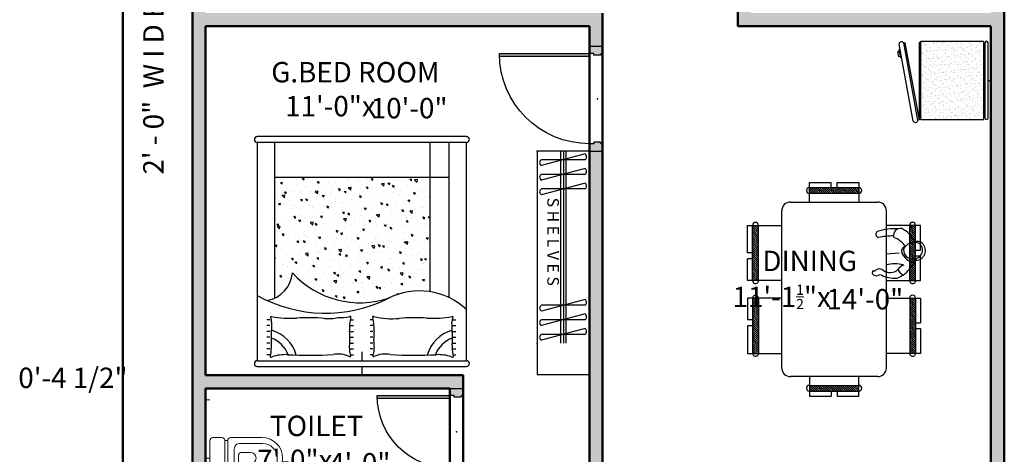
# Model space of a CAD drawing. Units: inches. Extents: x 4508 to 5907, y 877 to 1592.
# Tile 3 of 20: x 4536 to 4874, y 1182 to 1331. Entities that reach past the tile are written whole.
import ezdxf

# ---------------------------------------------------------------- set-up
doc = ezdxf.new("R2010")
doc.units = ezdxf.units.IN
doc.layers.get('DEFPOINTS').update_dxf_attribs({"color": 8})
for name, color, linetype, lineweight in [('A-ANNO-DIMS', 2, 'Continuous', 18), ('A-ANNO-TEXT', 7, 'Continuous', 25), ('A-DOOR', 4, 'Continuous', 25), ('A-FLOR-CASE', 30, 'Continuous', 25), ('A-FLOR-FIXT', 8, 'Continuous', 18), ('A-FURN', 24, 'Continuous', 18), ('A-WALL', 7, 'Continuous', 50), ('A-WALL-PATT', 8, 'Continuous', 13)]:
    doc.layers.add(name, color=color, linetype=linetype, lineweight=lineweight)
doc.layers.add('doors & windows', color=30, linetype='Continuous')
doc.layers.add('furniture', color=24, linetype='Continuous')
doc.styles.get("Standard").update_dxf_attribs({"font": 'arial.ttf'})
doc.dimstyles.new('details', dxfattribs={"dimtxt": 5, "dimasz": 2, "dimexe": 2, "dimexo": 3, "dimgap": 1, "dimtad": 0, "dimdec": 1, "dimzin": 0, "dimdsep": 46, "dimlunit": 4, "dimtxsty": 'Standard', "dimblk": 'ARCHTICK', "dimcen": 3, "dimclrd": 256, "dimclre": 256, "dimclrt": 256, "dimadec": 0, "dimazin": 0, "dimtfac": 0.5, "dimtdec": 1, "dimtofl": 0, "dimtmove": 0, "dimatfit": 3, "dimldrblk": 'CLOSEDBLANK', "dimfxl": 2, "dimtolj": 1, "dimtzin": 0, "dimlwd": -1, "dimlwe": -1, "dimarcsym": 0})
doc.dimstyles.new('text', dxfattribs={"dimtxt": 7, "dimasz": 0, "dimexe": 3, "dimexo": 3, "dimgap": 0, "dimtad": 1, "dimtih": 1, "dimtoh": 1, "dimzin": 3, "dimdsep": 46, "dimlunit": 4, "dimtxsty": 'Standard', "dimblk": 'CLOSEDBLANK', "dimcen": 3, "dimse1": 1, "dimse2": 1, "dimsd1": 1, "dimsd2": 1, "dimclrd": 256, "dimclre": 256, "dimclrt": 256, "dimadec": 0, "dimazin": 0, "dimtfac": 0.5, "dimtofl": 0, "dimtmove": 0, "dimatfit": 3, "dimfxl": 3, "dimtolj": 1, "dimtzin": 0, "dimlwd": -1, "dimlwe": -1, "dimarcsym": 0})
pattern_1 = [(45, (0, 0), (-0.3535534, 0.3535534), [])]

# ---------------------------------------------------------------- blocks, each defined once
blk = doc.blocks.new('refrigerator')
at = {"layer": 'furniture'}
h = blk.add_hatch(dxfattribs=at)
h.set_pattern_fill('AR-SAND', color=256, angle=-90, style=0)
h.set_pattern_definition([(307.5, (-13.5104, -1), (1.926824, 0.06299), [0, -1.52, 0, -1.7, 0, -1.625]), (277.5, (-13.5104, -1), (2.82215, -1.76978), [0, -0.82, 0, -1.37, 0, -0.525]), (237.5, (-13.5104, 0.23), (0.00566, -3.11414), [0, -0.5, 0, -1.8, 0, -2.35]), (227.5, (-13.5104, 0.23), (0.87768, -3.00613), [0, -0.25, 0, -1.18, 0, -1.35])])
h.paths.add_polyline_path([(13.6, -24.16), (13.6, -2.56), (-13.51, -2.56), (-13.51, -24.16)])
for p, q in [((0, -1), (0, 0)), ((-13.51, -2.56), (13.6, -2.56)), ((-13.51, -24.16), (-13.51, -2.56)), ((12.94, -1), (-12.94, -1)), ((12.94, -2), (-12.94, -2)), ((-12.41, -2), (-12.41, -2.56)), ((12.29, -2), (12.29, -2.56)), ((13.6, -2.56), (13.6, -24.16)), ((13.6, -24.16), (-13.51, -24.16)), ((-13.07, -24.59), (-13.07, -24.16)), ((13.26, -24.59), (-13.07, -24.59)), ((13.6, -24.61), (-12.95, -29.5)), ((13.7, -25.1), (-12.85, -29.99)), ((14.06, -26.73), (-12.49, -31.62)), ((13.07, -24.59), (13.26, -24.62)), ((13.26, -24.62), (13.07, -24.71)), ((13.26, -24.59), (13.26, -24.16)), ((13.6, -24.61), (13.7, -25.1)), ((-12.85, -29.99), (-12.95, -29.5)), ((-10.58, -31.27), (-10.49, -31.65)), ((-10.49, -31.65), (-7.79, -31.16)), ((-9.87, -32.01), (-9.97, -31.56)), ((-8.13, -31.69), (-9.87, -32.01)), ((-8.23, -31.24), (-8.13, -31.69)), ((-7.79, -31.16), (-7.88, -30.77))]:
    blk.add_line(p, q, dxfattribs=at)
for centre, radius, start, end in [((-12.94, -1.5), 0.5, 90, 270), ((12.94, -1.5), 0.5, 270, 90), ((13.58, -25.98), 0.888, 302.2332, 82.2568), ((-12.38, -30.74), 0.888, 122.2332, 262.2568)]:
    blk.add_arc(centre, radius, start, end, dxfattribs=at)
blk = doc.blocks.new('D1')
at = {"layer": 'doors & windows'}
h = blk.add_hatch(dxfattribs=at)
h.set_pattern_fill('DOTS', color=256, scale=2, angle=180, style=0)
h.set_pattern_definition([(180, (-2e-12, -4), (-0.0625, -0.125), [0, -0.125])])
h.paths.add_polyline_path([(2.5, 0), (3.5, 0), (3.5, 30.98, 0.008066), (2.5, 31)])
h = blk.add_hatch(dxfattribs=at)
h.set_pattern_fill('DOTS', color=256, scale=2, angle=180, style=0)
h.set_pattern_definition([(180, (0, -0.5), (-0.0625, -0.125), [0, -0.125])])
h.paths.add_polyline_path([(0, -4.5), (2.25, -4.5), (2.25, -4.25, 0.403966), (2.75, -3.75), (3, -3.75), (3, -1.5), (2.5, -1.5), (2.5, 0), (0, 0)])
h.paths.add_polyline_path([(36, -4.5), (36, 0), (33.5, 0), (33.5, -1.5), (33, -1.5), (33, -3.75), (33.25, -3.75, 0.403966), (33.75, -4.25), (33.75, -4.5)])
for p, q in [((0, 0), (0, -4.5)), ((36, 0), (36, -4.5))]:
    blk.add_line(p, q)
blk.add_lwpolyline([(3.5, 0), (3.5, 31), (2.5, 31), (2.5, 0)], close=True, dxfattribs=at)
for points in [[(3, -3.75), (3, -1.5), (2.5, -1.5), (2.5, 0), (0, 0)], [(33, -3.75), (33, -1.5), (33.5, -1.5), (33.5, 0), (36, 0)], [(0, -4.5), (2.25, -4.5)], [(36, -4.5), (33.75, -4.5)]]:
    blk.add_lwpolyline(points, dxfattribs=at)
for points in [[(2.25, -4.5), (2.25, -4.25, 0.403966), (2.75, -3.75), (3, -3.75)], [(33.75, -4.5), (33.75, -4.25, -0.403966), (33.25, -3.75), (33, -3.75)]]:
    blk.add_lwpolyline(points, format="xyb", dxfattribs=at)
at = {"layer": 'doors & windows', "ltscale": 6}
blk.add_arc((2.5, 0), 31, 0, 90, dxfattribs=at)
at = {"layer": 'doors & windows'}
blk.add_point((18, -2.75), dxfattribs=at)
blk = doc.blocks.new('*D32')
at = {"layer": 'DEFPOINTS', "color": 0, "transparency": 16777216}
for p in [(4685.1, 1328.7), (4669.73, 1208.7), (4671.99, 1208.7)]:
    blk.add_point(p, dxfattribs=at)
at = {"layer": 'A-ANNO-DIMS', "color": 0, "transparency": 16777216, "insert": (4669.73, 1300.51), "char_height": 7, "attachment_point": 5}
blk.add_mtext('\\A1;10\'-0"', dxfattribs=at)
blk = doc.blocks.new('_ClosedBlank')
at = {"color": 0, "lineweight": -2}
for p, q in [((-1, 0.17), (0, 0)), ((-1, 0.17), (-1, -0.17)), ((0, 0), (-1, -0.17))]:
    blk.add_line(p, q, dxfattribs=at)
blk = doc.blocks.new('*D33')
at = {"layer": 'DEFPOINTS', "color": 0, "transparency": 16777216}
for p in [(4731.74, 1297.56), (4599.74, 1268.7), (4731.74, 1268.7)]:
    blk.add_point(p, dxfattribs=at)
at = {"layer": 'A-ANNO-DIMS', "color": 0, "transparency": 16777216, "insert": (4642.67, 1307.03), "char_height": 7, "attachment_point": 5}
blk.add_mtext('\\A1;        G.BED ROOM\\P11\'-0"x', dxfattribs=at)
blk = doc.blocks.new('bed')
at = {"layer": 'furniture'}
h = blk.add_hatch(dxfattribs=at)
h.set_pattern_fill('AR-CONC', color=256, angle=-90, style=0)
h.set_pattern_definition([(320, (0, 2.38), (-0.6275, -7.1726), [0.75, -8.25]), (265, (0, 2.38), (7.5219, 1.3875), [0.6, -6.6]), (10.451, (-0.052, 1.782), (6.8944, -5.7851), [0.6374, -7.0114]), (316.184, (2, 2.38), (-1.6552, -10.6724), [1.125, -12.375]), (6.636, (1.862, 1.491), (9.7412, -9.3466), [0.9561, -10.5171]), (261.184, (2, 2.38), (9.7412, -9.3466), [0.9, -9.9]), (291, (1.5, 1.38), (-4.0262, -5.96907), [0.75, -8.25]), (236, (1.5, 1.38), (7.2515, -2.43315), [0.6, -6.6]), (341.451, (1.1645, 0.8826), (3.2253, -8.4022), [0.6374, -7.0114]), (307.5, (0, 2.38), (3.32894, -0.1216), [0, -6.52, 0, -6.7, 0, -6.625]), (277.5, (0, 2.38), (3.94412, -2.6307), [0, -3.82, 0, -6.37, 0, -2.525]), (237.5, (0, 4.61), (-0.22555, -5.33822), [0, -2.5, 0, -7.8, 0, -10.35]), (227.5, (0, 5.61), (1.00105, -5.83186), [0, -3.25, 0, -5.18, 0, -7.35])])
h.paths.add_polyline_path([(30.01, -68), (30.01, -26.5, 0.263043), (23.9, -35.15, 0.293424), (-9.18, -26.47, -0.156683), (-23.39, -28.72), (-23.39, -68)])
for p, q in [((0, -3), (0, 0)), ((36.01, -3), (-36.01, -3)), ((-36.01, -5), (-36.01, -80)), ((36.01, -5), (-36.01, -5)), ((0, -8), (0, -5)), ((36.01, -80), (36.01, -5)), ((-31.24, -7.07), (-32.24, -7.07)), ((-31.24, -9.07), (-32.24, -9.07)), ((-3.81, -7.07), (-2.81, -7.07)), ((-3.81, -9.07), (-2.81, -9.07)), ((3.89, -7.07), (2.89, -7.07)), ((3.89, -9.07), (2.89, -9.07)), ((31.63, -7.07), (32.63, -7.07)), ((31.63, -9.07), (32.63, -9.07)), ((-31.24, -11.07), (-32.24, -11.07)), ((-31.24, -13.07), (-32.24, -13.07)), ((-3.81, -11.07), (-2.81, -11.07)), ((-3.81, -13.07), (-2.81, -13.07)), ((3.89, -11.07), (2.89, -11.07)), ((3.89, -13.07), (2.89, -13.07)), ((31.63, -11.07), (32.63, -11.07)), ((31.63, -13.07), (32.63, -13.07)), ((-31.24, -15.07), (-32.24, -15.07)), ((-3.81, -15.07), (-2.81, -15.07)), ((3.89, -15.07), (2.89, -15.07)), ((31.63, -15.07), (32.63, -15.07)), ((-31.24, -17.07), (-32.24, -17.07)), ((-31.24, -19.07), (-32.24, -19.07)), ((-3.81, -17.07), (-2.81, -17.07)), ((-3.81, -19.07), (-2.81, -19.07)), ((3.89, -17.07), (2.89, -17.07)), ((3.89, -19.07), (2.89, -19.07)), ((31.63, -17.07), (32.63, -17.07)), ((31.63, -19.07), (32.63, -19.07)), ((-36.01, -80), (36.01, -80)), ((-36.01, -82), (36.01, -82))]:
    blk.add_line(p, q, dxfattribs=at)
at = {"layer": 'furniture', "ltscale": 5}
blk.add_line((-30.01, -26.66), (-30.01, -80), dxfattribs=at)
at = {"layer": 'furniture', "ltscale": 7}
blk.add_line((30.01, -80), (30.01, -26.5), dxfattribs=at)
at = {"layer": 'furniture', "ltscale": 0.3}
for p, q in [((-23.39, -80), (-23.39, -28.72)), ((-30.01, -68), (30.01, -68))]:
    blk.add_line(p, q, dxfattribs=at)
at = {"layer": 'furniture'}
for centre, radius, start, end in [((-35.95, -4), 1, 93.3831, 266.6169), ((35.95, -4), 1, 273.3831, 86.6169), ((-31.1, -6.57), 0.382, 35.8976, 208.6272), ((-44.44, -13.85), 14.82, 27.1629, 28.6272), ((-26.35, 6.68), 13.76, 251.1782, 273.3982), ((-8.03, 2.03), 9.29, 258.896, 294.7184), ((-4.03, -6.67), 0.282, 335.7259, 114.303), ((4.11, -6.67), 0.282, 65.697, 204.2741), ((8.12, 2.03), 9.29, 245.2816, 281.104), ((26.43, 6.68), 13.76, 266.6018, 288.8218), ((31.18, -6.57), 0.382, 331.3728, 144.1024), ((44.53, -13.85), 14.82, 151.3728, 152.8371), ((-46.76, -9.65), 15.72, 357.4804, 9.3956), ((-34.45, -3.51), 9.85, 289.8695, 338.9843), ((-34.45, -3.51), 12.47, 286.0319, 344.1205), ((-18.02, -163.6), 156.72, 87.0032, 92.7497), ((0.25, -8.8), 4.49, 159.0146, 186.273), ((-32.82, -12.44), 28.78, 354.3784, 6.273), ((3.22, -9.94), 7.68, 155.7259, 159.0146), ((-3.14, -9.94), 7.68, 20.9854, 24.2741), ((-0.17, -8.8), 4.49, 353.727, 20.9854), ((32.9, -12.44), 28.78, 173.727, 185.6216), ((18.1, -163.6), 156.72, 87.2503, 92.9968), ((34.54, -3.51), 12.47, 195.8795, 253.9681), ((34.54, -3.51), 9.85, 201.0157, 250.1305), ((46.84, -9.65), 15.72, 170.6044, 182.5196), ((-28.62, 31.03), 42.31, 266.4836, 266.6487), ((54.88, -13.16), 85.99, 178.1209, 183.3613), ((-54.8, -13.16), 85.99, 356.6387, 1.8791), ((28.7, 31.03), 42.31, 273.3513, 273.5164), ((12.28, -16.11), 16.48, 177.0317, 192.8678), ((-12.19, -16.11), 16.48, 347.1322, 2.9683), ((-31.05, -19.91), 0.291, 147.6219, 311.9343), ((-33.2, -18.55), 2.25, 327.6219, 339.2246), ((-34.13, -18.41), 3.18, 342.7809, 3.755), ((-24.4, -58.01), 38.42, 93.5164, 99.6766), ((-24.52, -56.06), 36.48, 86.4836, 93.5164), ((-18.49, 70.49), 90.23, 267.5921, 273.6329), ((-10.31, -44.95), 25.52, 75.952, 95.5452), ((-3.95, -19.99), 0.265, 231.9005, 52.8902), ((4.03, -19.99), 0.265, 127.1098, 308.0995), ((7.57, -34.68), 14.87, 87.3976, 103.1191), ((11.44, -34.81), 15.32, 84.694, 102.0355), ((18.57, 70.49), 90.23, 266.3671, 272.4079), ((24.6, -56.06), 36.48, 86.4836, 93.5164), ((24.48, -58.01), 38.42, 80.3234, 86.4836), ((31.13, -19.91), 0.291, 228.0657, 32.3781), ((34.21, -18.41), 3.18, 176.245, 197.2191), ((33.28, -18.55), 2.25, 200.7754, 212.3781), ((-19.79, -5.47), 23.53, 226.4061, 297.4441), ((12.51, -69.71), 48.38, 60.9345, 116.3227), ((0.6, -56.57), 31.65, 42.5874, 108.5034), ((34.61, -36.23), 10.76, 101.1719, 174.259), ((-35.95, -81), 1, 93.3831, 266.6169), ((35.95, -81), 1, 273.3831, 86.6169)]:
    blk.add_arc(centre, radius, start, end, dxfattribs=at)
blk = doc.blocks.new('hangers')
at = {"layer": 'furniture'}
for p, q in [((1, 7.5), (5, -7.5)), ((3, 7.5), (3, -7.5)), ((6, 7.5), (10, -7.5)), ((8, 7.5), (8, -7.5)), ((11, 7.5), (15, -7.5)), ((13, 7.5), (13, -7.5)), ((51, 7.5), (55, -7.5)), ((53, 7.5), (53, -7.5)), ((56, 7.5), (60, -7.5)), ((58, 7.5), (58, -7.5)), ((61, 7.5), (65, -7.5)), ((63, 7.5), (63, -7.5)), ((66, 1), (0, 1)), ((0, 0), (66, 0)), ((0, -1), (66, -1))]:
    blk.add_line(p, q, dxfattribs=at)
for centre, radius, start, end in [((2, 6.62), 1.33, 41.2884, 138.7116), ((7, 6.62), 1.33, 41.2884, 138.7116), ((12, 6.62), 1.33, 41.2884, 138.7116), ((52, 6.62), 1.33, 41.2884, 138.7116), ((57, 6.62), 1.33, 41.2884, 138.7116), ((62, 6.62), 1.33, 41.2884, 138.7116), ((4, -7.08), 1.08, 202.5549, 337.4451), ((9, -7.08), 1.08, 202.5549, 337.4451), ((14, -7.08), 1.08, 202.5549, 337.4451), ((54, -7.08), 1.08, 202.5549, 337.4451), ((59, -7.08), 1.08, 202.5549, 337.4451), ((64, -7.08), 1.08, 202.5549, 337.4451)]:
    blk.add_arc(centre, radius, start, end, dxfattribs=at)
for p in [(0, 9), (66, 9), (0, -9), (66, -9)]:
    blk.add_point(p, dxfattribs=at)
blk.add_text('S H E L V E S', height=4, dxfattribs=at).set_placement((16, -5.52))
blk = doc.blocks.new('*D34')
at = {"layer": 'DEFPOINTS', "color": 0, "transparency": 16777216}
for p in [(4683.74, 1178.32), (4683.74, 1175.99), (4599.74, 1170.14)]:
    blk.add_point(p, dxfattribs=at)
at = {"layer": 'A-ANNO-DIMS', "color": 0, "transparency": 16777216, "insert": (4630.42, 1185.46), "char_height": 7, "attachment_point": 5}
blk.add_mtext('\\A1;       TOILET\\P7\'-0"x', dxfattribs=at)
blk = doc.blocks.new('*D35')
at = {"layer": 'DEFPOINTS', "color": 0, "transparency": 16777216}
for p in [(4647.76, 1204.2), (4647.07, 1156.2), (4652.75, 1156.2)]:
    blk.add_point(p, dxfattribs=at)
at = {"layer": 'A-ANNO-DIMS', "color": 0, "transparency": 16777216, "insert": (4652.75, 1178.45), "char_height": 7, "attachment_point": 5}
blk.add_mtext('\\A1;4\'-0"', dxfattribs=at)
blk = doc.blocks.new('D2')
at = {"layer": 'doors & windows'}
h = blk.add_hatch(dxfattribs=at)
h.set_pattern_fill('DOTS', color=256, scale=2, angle=180, style=0)
h.set_pattern_definition([(180, (0, -4), (-0.0625, -0.125), [0, -0.125])])
h.paths.add_polyline_path([(2.5, 0), (3.5, 0), (3.5, 24.98, 0.010003), (2.5, 25)])
h = blk.add_hatch(dxfattribs=at)
h.set_pattern_fill('DOTS', color=256, scale=2, angle=180, style=0)
h.set_pattern_definition([(180, (0, 0), (-0.0625, -0.125), [0, -0.125])])
edge = h.paths.add_edge_path()
edge.add_line((27.5, 0), (27.5, -1.5))
edge.add_line((27.5, -1.5), (27, -1.5))
edge.add_line((27, -1.5), (27, -3.75))
edge.add_line((27, -3.75), (27.25, -3.75))
edge.add_arc((27.76, -3.74), 0.509, 181.0059, 268.9941)
edge.add_line((27.75, -4.25), (27.75, -4.5))
edge.add_line((27.75, -4.5), (30, -4.5))
edge.add_line((30, -4.5), (30, 0))
edge.add_line((30, 0), (27.5, 0))
edge = h.paths.add_edge_path()
edge.add_line((2.5, -1.5), (2.5, 0))
edge.add_line((2.5, 0), (0, 0))
edge.add_line((0, 0), (0, -4.5))
edge.add_line((0, -4.5), (2.25, -4.5))
edge.add_line((2.25, -4.5), (2.25, -4.25))
edge.add_arc((2.24, -3.74), 0.509, 271.0059, 358.9941)
edge.add_line((2.75, -3.75), (3, -3.75))
edge.add_line((3, -3.75), (3, -1.5))
edge.add_line((3, -1.5), (2.5, -1.5))
for p, q in [((0, 0), (0, -4.5)), ((30, 0), (30, -4.5))]:
    blk.add_line(p, q)
blk.add_lwpolyline([(3.5, 0), (3.5, 25), (2.5, 25), (2.5, 0)], close=True, dxfattribs=at)
for points in [[(3, -3.75), (3, -1.5), (2.5, -1.5), (2.5, 0), (0, 0)], [(27, -3.75), (27, -1.5), (27.5, -1.5), (27.5, 0), (30, 0)], [(0, -4.5), (2.25, -4.5)], [(30, -4.5), (27.75, -4.5)]]:
    blk.add_lwpolyline(points, dxfattribs=at)
for points in [[(2.25, -4.5), (2.25, -4.25, 0.403966), (2.75, -3.75), (3, -3.75)], [(27.75, -4.5), (27.75, -4.25, -0.403966), (27.25, -3.75), (27, -3.75)]]:
    blk.add_lwpolyline(points, format="xyb", dxfattribs=at)
at = {"layer": 'doors & windows', "ltscale": 6}
blk.add_arc((2.5, 0), 25, 0, 90, dxfattribs=at)
at = {"layer": 'doors & windows'}
blk.add_point((15, -2.25), dxfattribs=at)
blk = doc.blocks.new('commode')
for p, q in [((-7.09, 19.41), (-7.09, 8.61)), ((-5.09, 11.81), (-5.09, 19.57)), ((5.09, 11.81), (5.09, 19.57)), ((7.09, 19.41), (7.09, 8.61)), ((-2, 12.37), (-2, 15.37)), ((2, 12.37), (2, 15.37)), ((-1, 11.37), (1, 11.37)), ((-6.09, 7.61), (6.09, 7.61)), ((-6.09, 6.61), (-6.09, 7.61)), ((-3.15, 9.87), (3.15, 9.87)), ((6.09, 7.61), (6.09, 6.61)), ((-7.09, 2.5), (-7.09, 5.61)), ((-6.09, 6.61), (6.09, 6.61)), ((7.09, 2.5), (7.09, 5.61)), ((-20, 1.5), (-20, 0)), ((-6.09, 1.5), (6.09, 1.5)), ((0, 1.5), (0, 0)), ((20, 1.5), (20, 0))]:
    blk.add_line(p, q)
for centre, radius, start, end in [((0, 19.41), 7.09, 0, 180), ((0, 19.57), 5.09, 0, 180), ((0, 15.37), 2, 0, 180), ((-3.15, 11.81), 1.94, 180, 270), ((-1, 12.37), 1, 180, 270), ((1, 12.37), 1, 270, 0), ((3.15, 11.81), 1.94, 270, 0), ((-6.09, 8.61), 1, 180, 270), ((6.09, 8.61), 1, 270, 0), ((-6.09, 5.61), 1, 90, 180), ((6.09, 5.61), 1, 0, 90), ((-6.09, 2.5), 1, 180, 270), ((6.09, 2.5), 1, 270, 0)]:
    blk.add_arc(centre, radius, start, end)
blk = doc.blocks.new('*D46')
at = {"layer": 'DEFPOINTS', "color": 0, "transparency": 16777216}
for p in [(4736.24, 1231.48), (4736.24, 1219.56), (4869.74, 1215.47)]:
    blk.add_point(p, dxfattribs=at)
at = {"layer": 'A-ANNO-DIMS', "color": 0, "transparency": 16777216, "insert": (4797.8, 1241.47), "char_height": 7, "attachment_point": 5}
blk.add_mtext('\\A1;         DINING\\P11\'-1{\\H0.5x;\\S1/2;}"x', dxfattribs=at)
blk = doc.blocks.new('*D47')
at = {"layer": 'DEFPOINTS', "color": 0, "transparency": 16777216}
for p in [(4826.39, 1328.7), (4829.43, 1328.7), (4817.29, 1160.7)]:
    blk.add_point(p, dxfattribs=at)
at = {"layer": 'A-ANNO-DIMS', "color": 0, "transparency": 16777216, "insert": (4826.39, 1234.84), "char_height": 7, "attachment_point": 5}
blk.add_mtext('\\A1;14\'-0"', dxfattribs=at)
blk = doc.blocks.new('DT')
at = {"layer": 'furniture'}
h = blk.add_hatch(dxfattribs=at)
h.set_pattern_fill('ANSI31', color=256, scale=4, style=0)
h.set_pattern_definition(pattern_1)
h.paths.add_polyline_path([(-34, -8.5), (-32, -8.5), (-32, 8.5), (-34, 8.5)])
h.paths.add_polyline_path([(-2, 26), (-2, 28), (-21, 28), (-21, 26)])
h.paths.add_polyline_path([(23, 26), (23, 28), (4, 28), (4, 26)])
h.paths.add_polyline_path([(23, -28), (23, -26), (4, -26), (4, -28)])
h.paths.add_polyline_path([(-2, -28), (-2, -26), (-21, -26), (-21, -28)])
h = blk.add_hatch(dxfattribs=at)
h.set_pattern_fill('ANSI31', color=256, scale=4, style=0)
h.set_pattern_definition(pattern_1)
h.paths.add_polyline_path([(34, -8.5), (36, -8.5), (36, 8.5), (34, 8.5)])
at = {"layer": 'doors & windows'}
blk.add_line((-11.2, 18.15), (-11.59, 22.33), dxfattribs=at)
for centre, radius, start, end in [((-12.34, 27.96), 3.42, 2.8928, 134.5528), ((-12.78, 20.33), 7.67, 108.0153, 157.5724), ((-13.21, 28.75), 2.25, 132.7993, 210.1219), ((-11.2, 27.56), 3.95, 155.2349, 248.5051), ((-12.43, 27.51), 2.91, 359.7942, 144.0351), ((-12.53, 26.93), 3.05, 267.7788, 10.6507), ((-13.37, 28.03), 5.08, 289.2819, 356.6237), ((-9.72, 27.09), 1.31, 352.7443, 87.7525), ((-20.97, 8.73), 22.84, 41.647, 56.3067), ((-8.5, 17.23), 8.99, 125.6851, 158.6987), ((-12.08, 24.9), 1.7, 192.3382, 283.0231), ((2.64, 20.82), 10.42, 162.7002, 196.7262), ((-4.27, 24.65), 3.12, 193.5598, 239.9446), ((-6.9, 24.92), 3.16, 289.6374, 341.2911), ((-17.49, 22.83), 2.42, 170.002, 284.7527), ((1.32, 21.08), 21.14, 177.1977, 197.248), ((6.61, 20.49), 23.98, 180.1725, 192.6992), ((-8.79, 19.27), 4.03, 325.4363, 41.8446), ((-13.17, 20.91), 10.36, 330.7562, 358.8997), ((-6.62, 20.83), 3.81, 358.2671, 46.939), ((-4.02, 15.59), 2.01, 136.0875, 215.1077), ((-17.93, 15.53), 1.19, 217.214, 345.0614), ((-5.98, 13.86), 0.655, 315.9836, 61.7947), ((-5.73, 14.57), 2.04, 328.4119, 38.6474), ((-4.79, 14.1), 0.998, 224.0636, 323.687)]:
    blk.add_arc(centre, radius, start, end, dxfattribs=at)
at = {"layer": 'furniture'}
for p, q in [((-21, 29.75), (-21, 18)), ((-12.5, 29.75), (-21, 29.75)), ((-2, 28), (-21, 28)), ((-12.5, 28), (-12.5, 29.75)), ((-10.5, 28), (-10.5, 29.75)), ((-2, 29.75), (-10.5, 29.75)), ((-2, 18), (-2, 29.75)), ((4, 18), (4, 29.75)), ((4, 29.75), (12.5, 29.75)), ((4, 28), (23, 28)), ((12.5, 28), (12.5, 29.75)), ((14.5, 28), (14.5, 29.75)), ((14.5, 29.75), (23, 29.75)), ((23, 29.75), (23, 18)), ((-2, 26), (-21, 26)), ((4, 26), (23, 26)), ((28, 18), (-26, 18)), ((-29, -15), (-29, 15)), ((31, 15), (31, -15)), ((-35.75, 1), (-35.75, 8.5)), ((-35.75, 8.5), (-29, 8.5)), ((-34, -8.5), (-34, 8.5)), ((-32, -8.5), (-32, 8.5)), ((37.75, 8.5), (31, 8.5)), ((34, -8.5), (34, 8.5)), ((36, -8.5), (36, 8.5)), ((37.75, 1), (37.75, 8.5)), ((-34, 1), (-35.75, 1)), ((36, 1), (37.75, 1)), ((-34, -1), (-35.75, -1)), ((-35.75, -8.5), (-35.75, -1)), ((36, -1), (37.75, -1)), ((37.75, -8.5), (37.75, -1)), ((-29, -8.5), (-35.75, -8.5)), ((31, -8.5), (37.75, -8.5)), ((28, -18), (-26, -18)), ((-21, -29.75), (-21, -18)), ((-2, -18), (-2, -29.75)), ((4, -18), (4, -29.75)), ((23, -29.75), (23, -18)), ((-2, -26), (-21, -26)), ((4, -26), (23, -26)), ((-2, -28), (-21, -28)), ((-11.5, -29.75), (-21, -29.75)), ((-11.5, -28), (-11.5, -29.75)), ((-9.5, -28), (-9.5, -29.75)), ((-2, -29.75), (-9.5, -29.75)), ((4, -28), (23, -28)), ((4, -29.75), (11.5, -29.75)), ((11.5, -28), (11.5, -29.75)), ((13.5, -28), (13.5, -29.75)), ((13.5, -29.75), (23, -29.75))]:
    blk.add_line(p, q, dxfattribs=at)
for centre, radius, start, end in [((-21, 27), 1, 90, 270), ((-2, 27), 1, 270, 90), ((4, 27), 1, 90, 270), ((23, 27), 1, 270, 90), ((-26, 15), 3, 90, 180), ((28, 15), 3, 0, 90), ((-33, 8.5), 1, 0, 180), ((35, 8.5), 1, 0, 180), ((-33, -8.5), 1, 180, 0), ((35, -8.5), 1, 180, 0), ((-26, -15), 3, 180, 270), ((28, -15), 3, 270, 0), ((-21, -27), 1, 90, 270), ((-2, -27), 1, 270, 90), ((4, -27), 1, 90, 270), ((23, -27), 1, 270, 90)]:
    blk.add_arc(centre, radius, start, end, dxfattribs=at)
blk.add_point((1, 0), dxfattribs=at)
blk = doc.blocks.new('_ArchTick')
at = {"color": 0, "linetype": 'ByBlock', "const_width": 0.15}
blk.add_lwpolyline([(-0.5, -0.5), (0.5, 0.5)], dxfattribs=at)
blk = doc.blocks.new('*D52')
at = {"layer": 'A-ANNO-DIMS', "color": 0, "transparency": 16777216}
for p, q in [((4877.24, 1574.7), (4891.29, 1574.7)), ((4889.29, 1574.7), (4889.29, 1255.95)), ((4889.29, 926.7), (4889.29, 1245.46)), ((4877.24, 926.7), (4891.29, 926.7))]:
    blk.add_line(p, q, dxfattribs=at)
at = {"layer": 'DEFPOINTS', "color": 0, "transparency": 16777216}
for p in [(4874.24, 1574.7), (4874.24, 926.7), (4889.29, 926.7)]:
    blk.add_point(p, dxfattribs=at)
at = {"layer": 'A-ANNO-DIMS', "color": 0, "transparency": 16777216, "xscale": 2, "yscale": 2, "zscale": 2}
for p, rotation in [((4889.29, 1574.7), 90), ((4889.29, 926.7), 270)]:
    blk.add_blockref('_ArchTick', p, dxfattribs=dict(at, rotation=rotation))
at = {"layer": 'A-ANNO-DIMS', "color": 0, "transparency": 16777216, "insert": (4889.29, 1250.7), "char_height": 5, "attachment_point": 5, "rotation": 90}
blk.add_mtext("\\A1;54'", dxfattribs=at)
blk = doc.blocks.new('*D184')
at = {"layer": 'DEFPOINTS', "color": 0, "transparency": 16777216}
for p in [(4536.69, 1208.7), (4599.74, 1208.7), (4599.74, 1204.2)]:
    blk.add_point(p, dxfattribs=at)
at = {"layer": 'A-ANNO-DIMS', "transparency": 16777216, "insert": (4554.15, 1207.82), "char_height": 7, "attachment_point": 5}
blk.add_mtext('\\A1;0\'-4 1/2"', dxfattribs=at)

msp = doc.modelspace()

# ---------------------------------------------------------------- hatches: boundary and pattern name
at = {"layer": 'A-WALL-PATT'}
h = msp.add_hatch(color=256, dxfattribs=at)
h.dxf.hatch_style = 1
h.paths.add_polyline_path([(4874.237, 926.704), (4874.237, 1481.704), (4869.737, 1481.704), (4869.737, 1385.704), (4787.237, 1385.704), (4787.237, 1395.704), (4782.737, 1395.704), (4782.737, 1385.704), (4782.737, 1381.204), (4787.237, 1381.204), (4847.237, 1381.204), (4869.737, 1381.204), (4869.737, 1333.204), (4847.237, 1333.204), (4787.237, 1333.204), (4787.237, 1345.204), (4782.737, 1345.204), (4782.737, 1328.704), (4869.737, 1328.704), (4869.737, 935.704), (4736.237, 935.704), (4736.237, 961.204), (4731.737, 961.204), (4731.737, 931.204), (4711.737, 931.204), (4659.737, 931.204), (4659.737, 991.204), (4731.737, 991.204), (4736.237, 991.204), (4736.237, 1115.704), (4731.737, 1115.704), (4731.737, 995.704), (4629.737, 995.704), (4629.737, 991.204), (4655.237, 991.204), (4655.237, 926.704)])
h.paths.add_polyline_path([(4599.737, 1151.704), (4731.737, 1151.704), (4731.737, 1156.204), (4688.237, 1156.204), (4688.237, 1174.204), (4683.737, 1174.204), (4683.737, 1156.204), (4599.737, 1156.204), (4599.737, 1204.204), (4683.737, 1204.204), (4688.237, 1204.204), (4688.237, 1208.704), (4599.737, 1208.704), (4599.737, 1328.704), (4731.737, 1328.704), (4731.737, 1321.757), (4736.237, 1321.757), (4736.237, 1333.204), (4599.737, 1333.204), (4599.737, 1481.704), (4606.251, 1481.704), (4606.251, 1490.704), (4595.237, 1490.704), (4595.237, 991.204), (4599.737, 991.204), (4599.737, 995.704)])
h.paths.add_polyline_path([(4736.237, 1285.757), (4731.737, 1285.757), (4731.737, 1151.704), (4736.237, 1151.704)], flags=17)

# ---------------------------------------------------------------- linework, layer by layer
at = {"layer": 'A-FLOR-CASE'}
for p, q in [((4713.737, 1285.757), (4713.737, 1208.955)), ((4731.737, 1285.757), (4713.737, 1285.757)), ((4713.737, 1208.955), (4731.737, 1208.955))]:
    msp.add_line(p, q, dxfattribs=at)
at = {"layer": 'A-WALL'}
for p, q in [((4571.237, 1574.704), (4571.237, 926.704)), ((4595.237, 1574.704), (4595.237, 926.704)), ((4874.237, 1574.704), (4874.237, 926.704)), ((4782.737, 1328.704), (4782.737, 1385.704)), ((4736.237, 1333.204), (4736.237, 935.704)), ((4599.737, 1328.704), (4731.737, 1328.704)), ((4599.737, 1328.704), (4599.737, 1208.704)), ((4731.737, 1328.704), (4731.737, 995.704)), ((4782.737, 1328.704), (4869.737, 1328.704)), ((4869.737, 1328.704), (4869.737, 935.704)), ((4599.737, 1208.704), (4688.237, 1208.704)), ((4688.237, 1208.704), (4688.237, 1156.204)), ((4599.737, 1204.204), (4683.737, 1204.204)), ((4599.737, 1204.204), (4599.737, 1156.204)), ((4683.737, 1204.204), (4683.737, 1156.204))]:
    msp.add_line(p, q, dxfattribs=at)

# ---------------------------------------------------------------- block references
at = {"layer": 'A-DOOR', "xscale": -1, "rotation": 90}
for name, p in [('D1', (4731.737, 1321.757)), ('D2', (4683.737, 1204.204))]:
    msp.add_blockref(name, p, dxfattribs=at)
at = {"layer": 'A-FLOR-FIXT', "rotation": 270}
msp.add_blockref('refrigerator', (4869.737, 1310.058), dxfattribs=at)
at = {"layer": 'A-FLOR-FIXT', "xscale": -1, "rotation": 270}
msp.add_blockref('commode', (4599.737, 1180.204), dxfattribs=at)
at = {"layer": 'A-FURN'}
for name, p, rotation in [('bed', (4653.479, 1208.704), 180), ('hangers', (4722.737, 1285.757), 270), ('DT', (4815.803, 1239.229), 270)]:
    msp.add_blockref(name, p, dxfattribs=dict(at, rotation=rotation))

# ---------------------------------------------------------------- texts
at = {"layer": 'A-ANNO-TEXT'}
msp.add_text('2\' - 0"  W I D E   L A N E', height=7, rotation=90, dxfattribs=at).set_placement((4585.29, 1277.676))

# ---------------------------------------------------------------- dimensions: what is measured, and where the dimension line sits
at = {"layer": 'A-ANNO-DIMS'}
for base, p1, p2, dimstyle, override, picture, middle in [((4889.286, 926.704), (4874.237, 1574.704), (4874.237, 926.704), 'details', {"dimclrd": 0, "dimclre": 0, "dimclrt": 0}, '*D52', (4889.286, 1250.704)), ((4536.687, 1208.704), (4599.737, 1204.204), (4599.737, 1208.704), 'text', {"dimdec": 1, "dimlfac": 1, "dimrnd": 0, "dimzin": 1, "dimdsep": 46, "dimlunit": 4, "dimfrac": 2}, '*D184', (4554.146, 1207.823))]:
    dim = msp.add_linear_dim(base=base, p1=p1, p2=p2, angle=90, dimstyle=dimstyle, override=override, dxfattribs=at)
    dim.commit()
    dim.dimension.update_dxf_attribs({"geometry": picture, "text_midpoint": middle})
for base, p1, p2, text, picture, middle in [((4731.737, 1297.56), (4599.737, 1268.704), (4731.737, 1268.704), '        G.BED ROOM\\P<>x', '*D33', (4642.669, 1297.56)), ((4683.737, 1175.992), (4599.737, 1170.144), (4683.737, 1178.322), '       TOILET\\P<>x', '*D34', (4630.423, 1175.992))]:
    dim = msp.add_linear_dim(base=base, p1=p1, p2=p2, text=text, dimstyle='text', override={"dimclrd": 0, "dimclre": 0, "dimclrt": 0}, dxfattribs=at)
    dim.commit()
    dim.dimension.update_dxf_attribs({"geometry": picture, "text_midpoint": middle, "dimtype": 160})
for base, p1, p2, picture, middle in [((4669.729, 1208.704), (4685.102, 1328.704), (4671.987, 1208.704), '*D32', (4669.729, 1300.511)), ((4826.392, 1328.704), (4817.287, 1160.704), (4829.435, 1328.704), '*D47', (4826.392, 1234.845)), ((4652.752, 1156.204), (4647.757, 1204.204), (4647.074, 1156.204), '*D35', (4652.752, 1178.448))]:
    dim = msp.add_linear_dim(base=base, p1=p1, p2=p2, angle=90, dimstyle='text', override={"dimclrd": 0, "dimclre": 0, "dimclrt": 0}, dxfattribs=at)
    dim.commit()
    dim.dimension.update_dxf_attribs({"geometry": picture, "text_midpoint": middle, "dimtype": 160})
dim = msp.add_linear_dim(base=(4736.237, 1231.478), p1=(4869.737, 1215.473), p2=(4736.237, 1219.564), angle=180, text='         DINING\\P<>x', dimstyle='text', override={"dimclrd": 0, "dimclre": 0, "dimclrt": 0}, dxfattribs=at)
dim.commit()
dim.dimension.update_dxf_attribs({"geometry": '*D46', "text_midpoint": (4797.803, 1231.478), "dimtype": 160})

doc.saveas('drawing.dxf')
